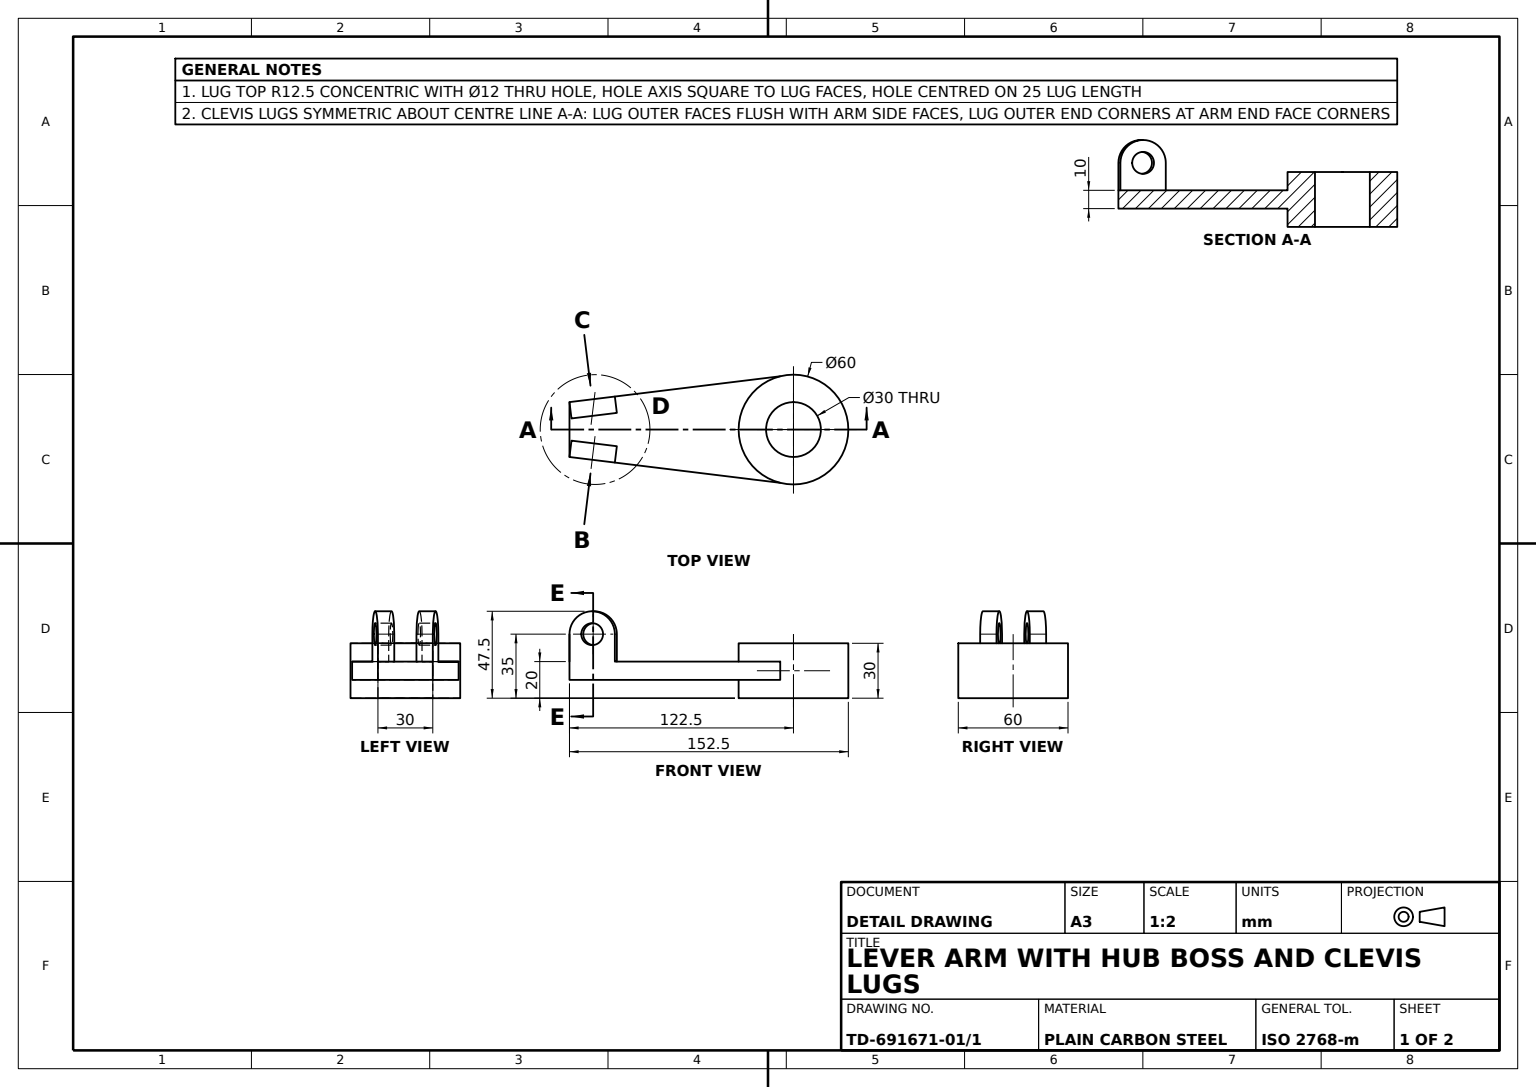
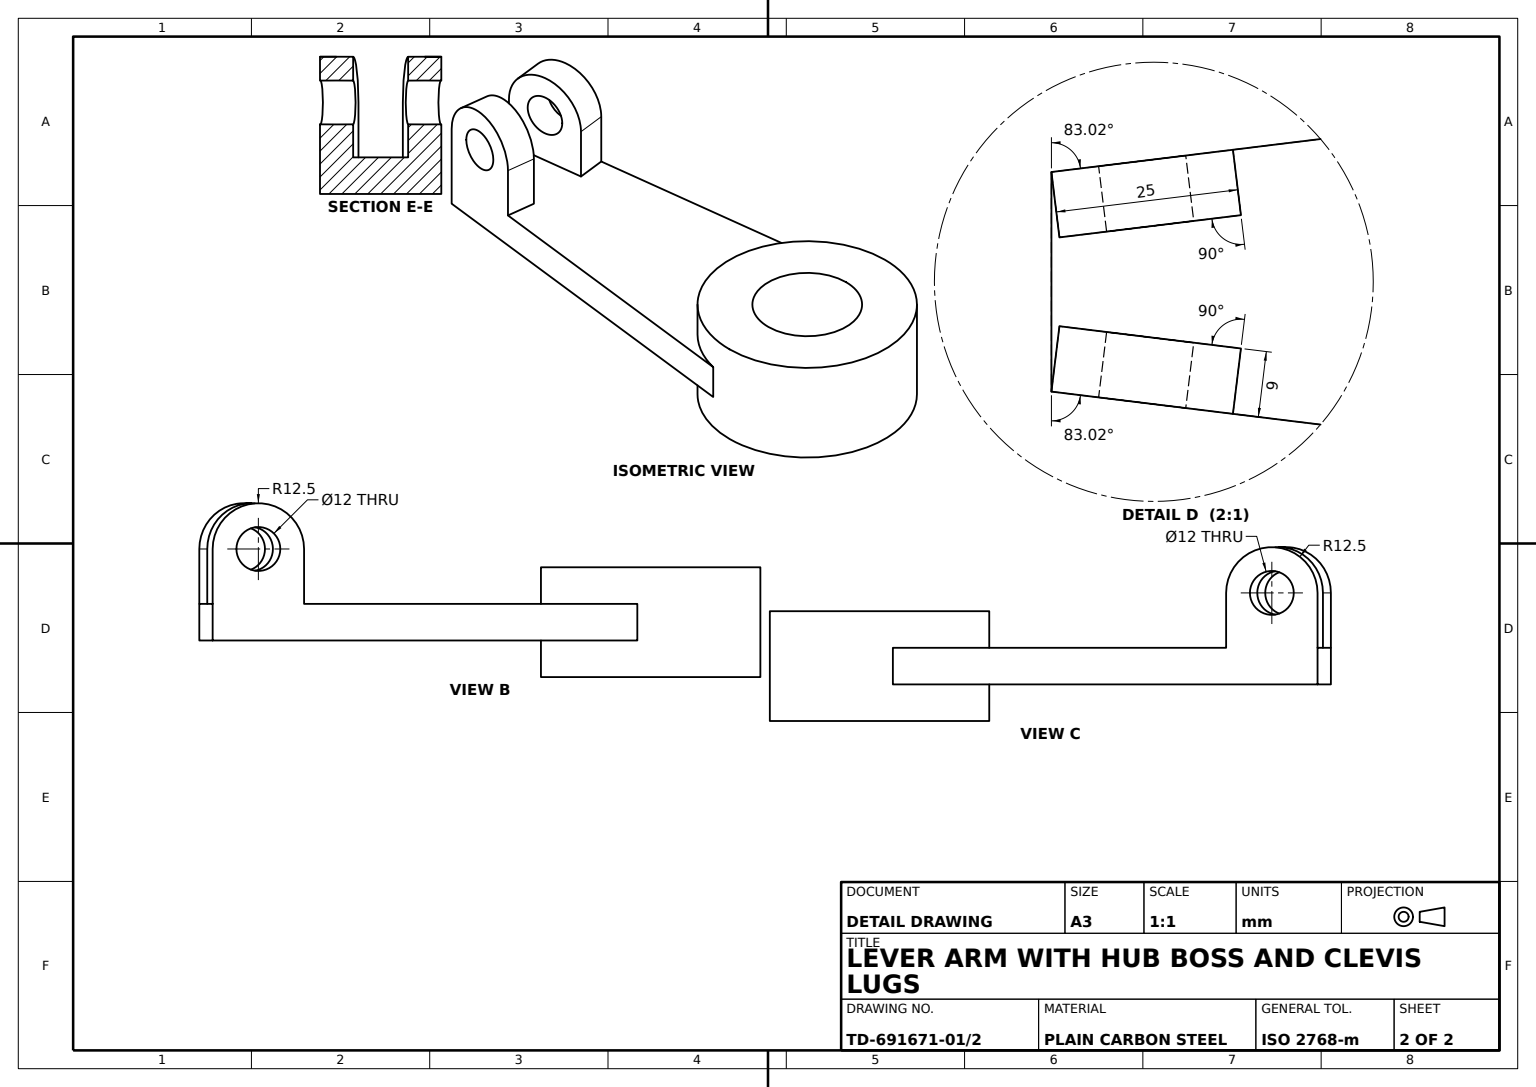
from build123d import *

# Parameters (mm, degrees)
HUB_PROFILE_SKETCH_R   = 30
HUB_60_DEPTH           = 20
LEVER_ARM_DEPTH        = 10
HUB_START              = 20
HUB_EXTENSION_SKETCH_R = 30
HUB_EXTENSION_DEPTH    = 20
CLEVIS_LUG_SKETCH_R    = 6
CLEVIS_LUG_DEPTH       = 9
HUB_RECESS_SKETCH_R    = 30
HUB_RECESS_CUT_DEPTH   = 10
BORE_SKETCH_R          = 15
HUB_BORE_30_DEPTH      = 46


with BuildPart() as part:
    # Hub Profile Sketch → Hub Ø60 (new body)
    with BuildSketch(Plane(origin=(0, 0, 0), x_dir=(1, 0, 0), z_dir=(0, 1, 0))):
        with Locations(Location((0, 0, 0), (0, 0, 270))):
            Circle(HUB_PROFILE_SKETCH_R)
    extrude(amount=HUB_60_DEPTH)

    # Arm Profile Sketch → Lever Arm (add)
    with BuildSketch(Plane(origin=(0, 0, 0), x_dir=(1, 0, 0), z_dir=(0, 1, 0))):
        with BuildLine():
            Line((-122.5, 0), (-30, 0))
            ThreePointArc((-30, 0), (-23.63421499, 18.477658992), (-7.238407879, 29.113664341))
            Line((-7.238407879, 29.113664341), (-122.5, 15))
            Line((-122.5, 15), (-122.5, 0))
        make_face()
        with BuildLine():
            ThreePointArc((-7.238407879, -29.113664341), (-23.63421499, -18.477658992), (-30, 0))
            Line((-30, 0), (-122.5, 0))
            Line((-122.5, 0), (-122.5, -15))
            Line((-122.5, -15), (-7.238407879, -29.113664341))
        make_face()
    extrude(amount=LEVER_ARM_DEPTH)

    # Hub Extension Sketch → Hub Extension (add)
    with BuildSketch(Plane.XZ.offset(HUB_START)):
        with Locations(Location((0, 0, 0), (0, 0, 270))):
            Circle(HUB_EXTENSION_SKETCH_R)
    extrude(amount=-HUB_EXTENSION_DEPTH)

    # Clevis Lug Sketch → Clevis Lug (add)
    with BuildSketch(Plane(origin=(-3.619203939, 0, -29.556832171), x_dir=(-0.9925863886954069, 0, 0.12154119045249893), z_dir=(-0.12154119045249893, 0, -0.9925863886954069))):
        with BuildLine():
            Line((119.768714758, 0), (119.768714758, 25))
            ThreePointArc((119.768714758, 25), (107.268714758, 37.5), (94.768714758, 25))
            Line((94.768714758, 25), (94.768714758, 0))
            Line((94.768714758, 0), (119.768714758, 0))
        make_face()
        with Locations((107.268714758, 25)):
            Circle(CLEVIS_LUG_SKETCH_R, mode=Mode.SUBTRACT)
    extrude(amount=-CLEVIS_LUG_DEPTH)

    # Clevis Lug Mirror: part across plane


with BuildPart() as part_1:
    add(part.part)
    add(part.part.mirror(Plane.XY))

    # Hub Recess Sketch → Hub Recess Cut (cut)
    with BuildSketch(Plane(origin=(0, -20, 0), x_dir=(-1, 0, 0), z_dir=(0, -1, 0))):
        with Locations(Location((0, 0, 0), (0, 0, 90))):
            Circle(HUB_RECESS_SKETCH_R)
    extrude(amount=-HUB_RECESS_CUT_DEPTH, mode=Mode.SUBTRACT)

    # Bore Sketch → Hub Bore Ø30 (cut)
    with BuildSketch(Plane(origin=(0, -10, 0), x_dir=(-1, 0, 0), z_dir=(0, -1, 0))):
        with Locations(Location((0, 0, 0), (0, 0, 90))):
            Circle(BORE_SKETCH_R)
    extrude(amount=-HUB_BORE_30_DEPTH, mode=Mode.SUBTRACT)


solid = part_1.part
